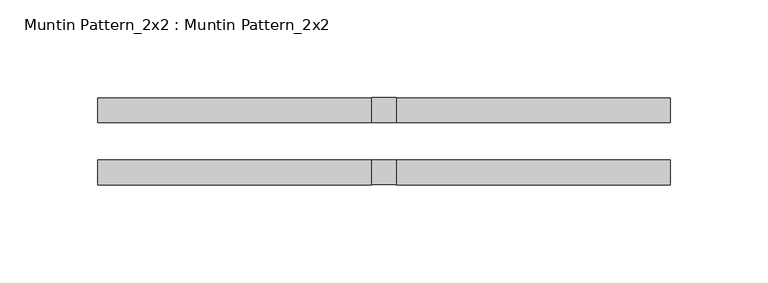
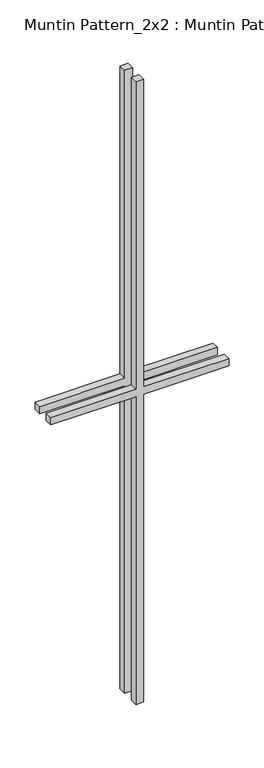
"""IFC4 building model written with IfcOpenShell, lengths in millimetres: proxy geometry, Muntin Pattern_2x2 : Muntin Pattern_2x2."""

from ifc_helpers import new_model, si_unit, frame, origin, place, context, project, spatial, polyline, outline, extrude, source, transform, mapped, element, save


def muntin_pattern_2x2_muntin_pattern_2x2_0e1f1e2d(model_context):
    return source(origin(), model_context, "Body", "SweptSolid", [
        extrude(outline(polyline([(546.1, -6.35), (546.1, -146.05), (533.4, -146.05), (533.4, -6.35), (0.0, -6.35), (0.0, 6.35), (533.4, 6.35), (533.4, 146.05), (546.1, 146.05), (546.1, 6.35), (1079.5, 6.35), (1079.5, -6.35), (546.1, -6.35)])), frame((0.0, 9.525, 0.0), z_axis=(0.0, 1.0, 0.0), x_axis=(0.0, 0.0, 1.0)), (0.0, 0.0, 1.0), 12.7),
        extrude(outline(polyline([(546.1, -6.35), (546.1, -146.05), (533.4, -146.05), (533.4, -6.35), (0.0, -6.35), (0.0, 6.35), (533.4, 6.35), (533.4, 146.05), (546.1, 146.05), (546.1, 6.35), (1079.5, 6.35), (1079.5, -6.35), (546.1, -6.35)])), frame((0.0, -22.225, 0.0), z_axis=(0.0, 1.0, 0.0), x_axis=(0.0, 0.0, 1.0)), (0.0, 0.0, 1.0), 12.7),
    ])


if __name__ == "__main__":
    model = new_model("IFC4")
    model_context = context("Model", 3, world=origin())
    ifc_project = project(units=[si_unit("LENGTHUNIT", "METRE", prefix="MILLI")], contexts=[model_context])
    site = spatial("IfcSite", under=ifc_project)
    building = spatial("IfcBuilding", under=site)
    placement = place(None, origin())
    muntin_pattern_2x2_muntin_pattern_2x2_shape = muntin_pattern_2x2_muntin_pattern_2x2_0e1f1e2d(model_context)
    element("IfcBuildingElementProxy", 1, Name="Muntin Pattern_2x2 : Muntin Pattern_2x2", ObjectType="Muntin Pattern_2x2 : Muntin Pattern_2x2", at=placement, inside=building, context=model_context, shape_type="MappedRepresentation", body=[
        mapped(muntin_pattern_2x2_muntin_pattern_2x2_shape, transform((0.0, 0.0, 0.0), x_axis=(1.0, 0.0, 0.0), y_axis=(0.0, 1.0, 0.0), z_axis=(0.0, 0.0, 1.0))),
    ])
    save(model, "model.ifc")

# Revit data of these elements
# Type "Muntin Pattern_2x2 : Muntin Pattern_2x2"
#   Width [instance default] = 4' - 0"
#   Thickness = 0' - 0 1/2"
#   Height [instance default] = 4' - 0"
#   Distance = 0' - 0 3/4"
#   Interior Material [instance default] = none
#   Exterior Material [instance default] = none
#   Default Elevation = 0
# Element 1 (IfcBuildingElementProxy, "Muntin Pattern_2x2 : Muntin Pattern_2x2")
#   Width = 0' - 11 1/2"
#   Height = 3' - 6 1/2"
#   Interior Material = Wood - Stained
#   Exterior Material = Clad - White
#   Materials on its faces: "Clad - White", "Wood - Stained"
# Materials
#   "Clad - White": class "Wood", colour RGB 242 242 238, transparency 0, Cost = 0
#   "Wood - Stained": class "Wood", colour RGB 224 178 126, transparency 0, Cost = 0
